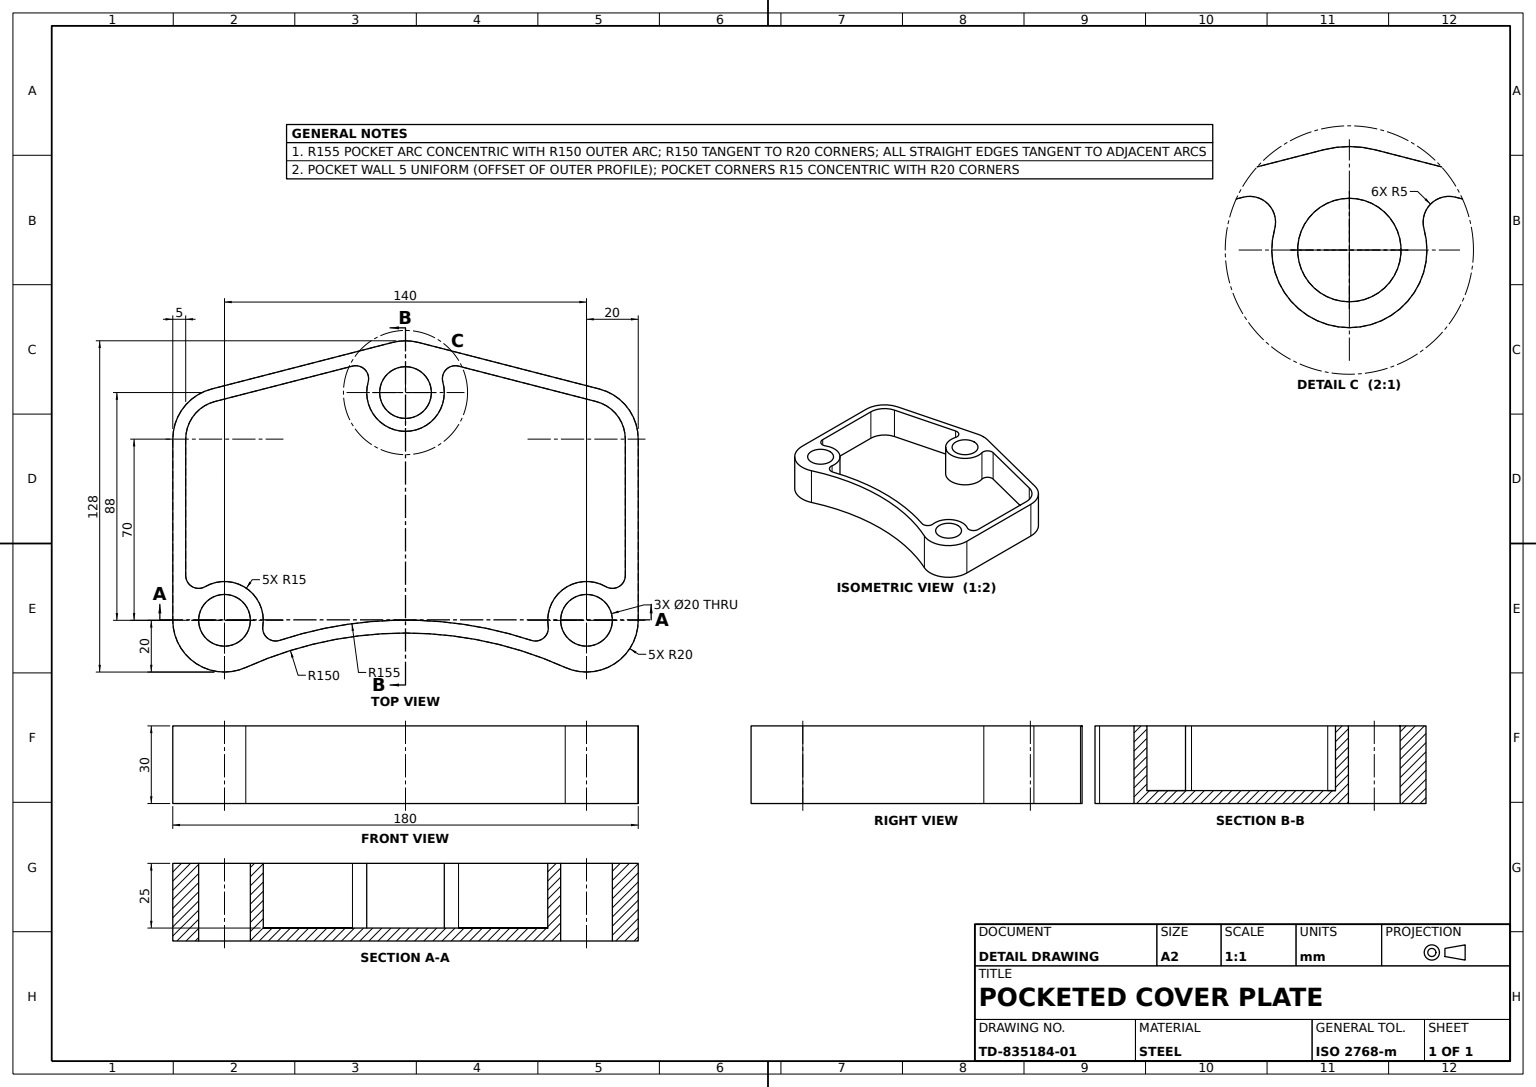
from build123d import *

# Parameters (mm, degrees)
BASE_PLATE_PROFILE_SKETCH_R = 10
BASE_PLATE_30MM_DEPTH       = 30
POCKET_25MM_DEEP_DEPTH      = 25


with BuildPart() as part:
    # Base Plate Profile Sketch → Base Plate 30mm (new body)
    with BuildSketch(Plane(origin=(0, 0, 0), x_dir=(1, 0, 0), z_dir=(0, 1, 0))):
        with BuildLine():
            Line((-74.980820796, 1.369858652), (-4.980820796, 19.369858652))
            ThreePointArc((-4.980820796, 19.369858652), (0, 20), (4.980820796, 19.369858652))
            Line((4.980820796, 19.369858652), (74.980820796, 1.369858652))
            ThreePointArc((74.980820796, 1.369858652), (85.80532214, -5.74472391), (90, -18))
            Line((90, -18), (90, -88))
            ThreePointArc((90, -88), (80.846522891, -104.803361008), (61.764705882, -106.225803982))
            ThreePointArc((61.764705882, -106.225803982), (0, -92.919333848), (-61.764705882, -106.225803982))
            ThreePointArc((-61.764705882, -106.225803982), (-80.846522891, -104.803361008), (-90, -88))
            Line((-90, -88), (-90, -18))
            ThreePointArc((-90, -18), (-85.80532214, -5.74472391), (-74.980820796, 1.369858652))
        make_face()
        with Locations(Location((0, 0, 0), (0, 0, 270))):
            Circle(BASE_PLATE_PROFILE_SKETCH_R, mode=Mode.SUBTRACT)
        with Locations(Location((-70, -88, 0), (0, 0, 270))):
            Circle(BASE_PLATE_PROFILE_SKETCH_R, mode=Mode.SUBTRACT)
        with Locations(Location((70, -88, 0), (0, 0, 270))):
            Circle(BASE_PLATE_PROFILE_SKETCH_R, mode=Mode.SUBTRACT)
    extrude(amount=BASE_PLATE_30MM_DEPTH)

    # Pocket Profile Sketch → Pocket 25mm Deep (cut)
    with BuildSketch(Plane(origin=(0, 30, 0), x_dir=(1, 0, 0), z_dir=(0, 1, 0))):
        with BuildLine():
            Line((-85, -18), (-85, -70.679491924))
            ThreePointArc((-85, -70.679491924), (-82.5, -75.009618943), (-77.5, -75.009618943))
            ThreePointArc((-77.5, -75.009618943), (-61.541849411, -75.612115249), (-55.170564121, -90.255622199))
            ThreePointArc((-55.170564121, -90.255622199), (-53.453138568, -94.827801509), (-48.657811989, -95.75474119))
            ThreePointArc((-48.657811989, -95.75474119), (0, -87.919333848), (48.657811989, -95.75474119))
            ThreePointArc((48.657811989, -95.75474119), (53.453138568, -94.827801509), (55.170564121, -90.255622199))
            ThreePointArc((55.170564121, -90.255622199), (61.541849411, -75.612115249), (77.5, -75.009618943))
            ThreePointArc((77.5, -75.009618943), (82.5, -75.009618943), (85, -70.679491924))
            Line((85, -70.679491924), (85, -18))
            ThreePointArc((85, -18), (81.853991605, -8.808542933), (73.735615597, -3.472606011))
            Line((73.735615597, -3.472606011), (20.510405257, 10.213876648))
            ThreePointArc((20.510405257, 10.213876648), (15.694105243, 8.871023652), (14.448900044, 4.028558989))
            ThreePointArc((14.448900044, 4.028558989), (0, -15), (-14.448900044, 4.028558989))
            ThreePointArc((-14.448900044, 4.028558989), (-15.694105243, 8.871023652), (-20.510405257, 10.213876648))
            Line((-20.510405257, 10.213876648), (-73.735615597, -3.472606011))
            ThreePointArc((-73.735615597, -3.472606011), (-81.853991605, -8.808542933), (-85, -18))
        make_face()
    extrude(amount=-POCKET_25MM_DEEP_DEPTH, mode=Mode.SUBTRACT)


solid = part.part
